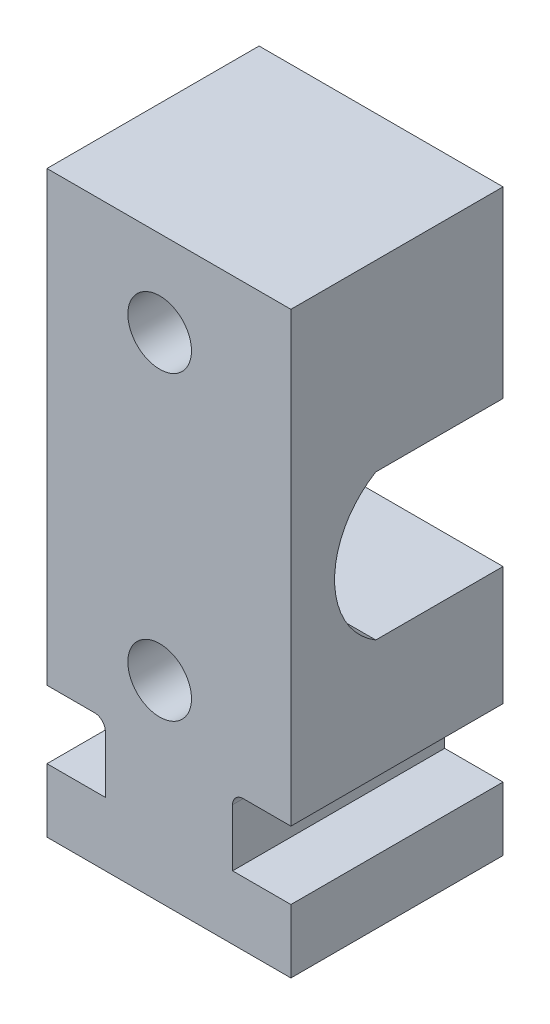
ISO-10303-21;
HEADER;
FILE_DESCRIPTION(('STEP AP214'),'2;1');
FILE_NAME('part.step','',(''),(''),'','','');
FILE_SCHEMA(('AUTOMOTIVE_DESIGN { 1 0 10303 214 1 1 1 1 }'));
ENDSEC;
DATA;
#1=APPLICATION_CONTEXT('core data for automotive mechanical design processes');
#2=APPLICATION_PROTOCOL_DEFINITION('international standard','automotive_design',2000,#1);
#3=PRODUCT_CONTEXT('',#1,'mechanical');
#4=PRODUCT('Part','Part','',(#3));
#5=PRODUCT_RELATED_PRODUCT_CATEGORY('part','',(#4));
#6=PRODUCT_DEFINITION_FORMATION('','',#4);
#7=PRODUCT_DEFINITION_CONTEXT('part definition',#1,'design');
#8=PRODUCT_DEFINITION('design','',#6,#7);
#9=PRODUCT_DEFINITION_SHAPE('','',#8);
#10=(LENGTH_UNIT() NAMED_UNIT(*) SI_UNIT(.MILLI.,.METRE.));
#11=(NAMED_UNIT(*) PLANE_ANGLE_UNIT() SI_UNIT($,.RADIAN.));
#12=(NAMED_UNIT(*) SI_UNIT($,.STERADIAN.) SOLID_ANGLE_UNIT());
#13=UNCERTAINTY_MEASURE_WITH_UNIT(LENGTH_MEASURE(1.E-05),#10,'distance_accuracy_value','');
#14=(GEOMETRIC_REPRESENTATION_CONTEXT(3) GLOBAL_UNCERTAINTY_ASSIGNED_CONTEXT((#13)) GLOBAL_UNIT_ASSIGNED_CONTEXT((#10,
#11,#12)) REPRESENTATION_CONTEXT('',''));
#15=CARTESIAN_POINT('',(0.,0.,0.));
#16=DIRECTION('',(0.,0.,1.));
#17=DIRECTION('',(1.,0.,0.));
#18=AXIS2_PLACEMENT_3D('',#15,#16,#17);
#19=CARTESIAN_POINT('',(115.,0.,100.));
#20=DIRECTION('',(-1.,0.,0.));
#21=DIRECTION('',(0.,0.,1.));
#22=AXIS2_PLACEMENT_3D('',#19,#20,#21);
#23=PLANE('',#22);
#24=DIRECTION('',(0.,0.,-1.));
#25=VECTOR('',#24,1.);
#26=CARTESIAN_POINT('',(115.,118.,100.));
#27=LINE('',#26,#25);
#28=CARTESIAN_POINT('',(115.,118.,60.));
#29=VERTEX_POINT('',#28);
#30=CARTESIAN_POINT('',(115.,118.,0.));
#31=VERTEX_POINT('',#30);
#32=EDGE_CURVE('E57',#29,#31,#27,.T.);
#33=ORIENTED_EDGE('',*,*,#32,.F.);
#34=CARTESIAN_POINT('',(115.,152.29480502863,39.4119853300948));
#35=DIRECTION('',(-1.,0.,0.));
#36=DIRECTION('',(0.,0.,1.));
#37=AXIS2_PLACEMENT_3D('',#34,#35,#36);
#38=CIRCLE('',#37,40.);
#39=CARTESIAN_POINT('',(115.,186.589610057261,60.));
#40=VERTEX_POINT('',#39);
#41=EDGE_CURVE('E58',#40,#29,#38,.F.);
#42=ORIENTED_EDGE('',*,*,#41,.F.);
#43=DIRECTION('',(0.,0.,1.));
#44=VECTOR('',#43,1.);
#45=CARTESIAN_POINT('',(115.,186.589610057261,100.));
#46=LINE('',#45,#44);
#47=CARTESIAN_POINT('',(115.,186.589610057261,0.));
#48=VERTEX_POINT('',#47);
#49=EDGE_CURVE('E180',#48,#40,#46,.T.);
#50=ORIENTED_EDGE('',*,*,#49,.F.);
#51=DIRECTION('',(0.,1.,0.));
#52=VECTOR('',#51,1.);
#53=CARTESIAN_POINT('',(115.,0.,0.));
#54=LINE('',#53,#52);
#55=CARTESIAN_POINT('',(115.,273.,0.));
#56=VERTEX_POINT('',#55);
#57=EDGE_CURVE('E165',#48,#56,#54,.T.);
#58=ORIENTED_EDGE('',*,*,#57,.T.);
#59=DIRECTION('',(0.,0.,-1.));
#60=VECTOR('',#59,1.);
#61=CARTESIAN_POINT('',(115.,273.,100.));
#62=LINE('',#61,#60);
#63=CARTESIAN_POINT('',(115.,273.,100.));
#64=VERTEX_POINT('',#63);
#65=EDGE_CURVE('E279',#64,#56,#62,.T.);
#66=ORIENTED_EDGE('',*,*,#65,.F.);
#67=DIRECTION('',(0.,1.,0.));
#68=VECTOR('',#67,1.);
#69=CARTESIAN_POINT('',(115.,0.,100.));
#70=LINE('',#69,#68);
#71=CARTESIAN_POINT('',(115.,62.,100.));
#72=VERTEX_POINT('',#71);
#73=EDGE_CURVE('E240',#72,#64,#70,.T.);
#74=ORIENTED_EDGE('',*,*,#73,.F.);
#75=DIRECTION('',(0.,0.,-1.));
#76=VECTOR('',#75,1.);
#77=CARTESIAN_POINT('',(115.,62.,100.));
#78=LINE('',#77,#76);
#79=CARTESIAN_POINT('',(115.,62.,0.));
#80=VERTEX_POINT('',#79);
#81=EDGE_CURVE('E278',#72,#80,#78,.T.);
#82=ORIENTED_EDGE('',*,*,#81,.T.);
#83=EDGE_CURVE('E172',#80,#31,#54,.T.);
#84=ORIENTED_EDGE('',*,*,#83,.T.);
#85=EDGE_LOOP('',(#33,#42,#50,#58,#66,#74,#82,#84));
#86=FACE_BOUND('',#85,.T.);
#87=ADVANCED_FACE('F41',(#86),#23,.F.);
#88=CARTESIAN_POINT('',(0.,0.,100.));
#89=DIRECTION('',(-1.,0.,0.));
#90=DIRECTION('',(0.,0.,1.));
#91=AXIS2_PLACEMENT_3D('',#88,#89,#90);
#92=PLANE('',#91);
#93=CARTESIAN_POINT('',(0.,152.29480502863,39.4119853300948));
#94=DIRECTION('',(-1.,0.,0.));
#95=DIRECTION('',(0.,0.,1.));
#96=AXIS2_PLACEMENT_3D('',#93,#94,#95);
#97=CIRCLE('',#96,40.);
#98=CARTESIAN_POINT('',(0.,186.589610057261,60.));
#99=VERTEX_POINT('',#98);
#100=CARTESIAN_POINT('',(0.,118.,60.));
#101=VERTEX_POINT('',#100);
#102=EDGE_CURVE('E11',#99,#101,#97,.F.);
#103=ORIENTED_EDGE('',*,*,#102,.T.);
#104=DIRECTION('',(0.,0.,-1.));
#105=VECTOR('',#104,1.);
#106=CARTESIAN_POINT('',(0.,118.,100.));
#107=LINE('',#106,#105);
#108=CARTESIAN_POINT('',(0.,118.,0.));
#109=VERTEX_POINT('',#108);
#110=EDGE_CURVE('E181',#101,#109,#107,.T.);
#111=ORIENTED_EDGE('',*,*,#110,.T.);
#112=DIRECTION('',(0.,1.,0.));
#113=VECTOR('',#112,1.);
#114=CARTESIAN_POINT('',(0.,0.,0.));
#115=LINE('',#114,#113);
#116=CARTESIAN_POINT('',(0.,62.,0.));
#117=VERTEX_POINT('',#116);
#118=EDGE_CURVE('E269',#117,#109,#115,.T.);
#119=ORIENTED_EDGE('',*,*,#118,.F.);
#120=DIRECTION('',(0.,0.,-1.));
#121=VECTOR('',#120,1.);
#122=CARTESIAN_POINT('',(0.,62.,100.));
#123=LINE('',#122,#121);
#124=CARTESIAN_POINT('',(0.,62.,100.));
#125=VERTEX_POINT('',#124);
#126=EDGE_CURVE('E274',#125,#117,#123,.T.);
#127=ORIENTED_EDGE('',*,*,#126,.F.);
#128=DIRECTION('',(0.,1.,0.));
#129=VECTOR('',#128,1.);
#130=CARTESIAN_POINT('',(0.,0.,100.));
#131=LINE('',#130,#129);
#132=CARTESIAN_POINT('',(0.,273.,100.));
#133=VERTEX_POINT('',#132);
#134=EDGE_CURVE('E237',#125,#133,#131,.T.);
#135=ORIENTED_EDGE('',*,*,#134,.T.);
#136=DIRECTION('',(0.,0.,-1.));
#137=VECTOR('',#136,1.);
#138=CARTESIAN_POINT('',(0.,273.,100.));
#139=LINE('',#138,#137);
#140=CARTESIAN_POINT('',(0.,273.,0.));
#141=VERTEX_POINT('',#140);
#142=EDGE_CURVE('E277',#133,#141,#139,.T.);
#143=ORIENTED_EDGE('',*,*,#142,.T.);
#144=CARTESIAN_POINT('',(0.,186.589610057261,0.));
#145=VERTEX_POINT('',#144);
#146=EDGE_CURVE('E267',#145,#141,#115,.T.);
#147=ORIENTED_EDGE('',*,*,#146,.F.);
#148=DIRECTION('',(0.,0.,1.));
#149=VECTOR('',#148,1.);
#150=CARTESIAN_POINT('',(0.,186.589610057261,100.));
#151=LINE('',#150,#149);
#152=EDGE_CURVE('E185',#145,#99,#151,.T.);
#153=ORIENTED_EDGE('',*,*,#152,.T.);
#154=EDGE_LOOP('',(#103,#111,#119,#127,#135,#143,#147,#153));
#155=FACE_BOUND('',#154,.T.);
#156=ADVANCED_FACE('F362',(#155),#92,.T.);
#157=CARTESIAN_POINT('',(0.,0.,0.));
#158=DIRECTION('',(0.,0.,1.));
#159=DIRECTION('',(1.,0.,0.));
#160=AXIS2_PLACEMENT_3D('',#157,#158,#159);
#161=PLANE('',#160);
#162=CARTESIAN_POINT('',(53.1264875684002,90.5995775376906,0.));
#163=DIRECTION('',(0.,0.,1.));
#164=DIRECTION('',(1.,0.,0.));
#165=AXIS2_PLACEMENT_3D('',#162,#163,#164);
#166=CIRCLE('',#165,15.);
#167=CARTESIAN_POINT('',(68.1264875684002,90.5995775376906,0.));
#168=VERTEX_POINT('',#167);
#169=EDGE_CURVE('E198',#168,#168,#166,.T.);
#170=ORIENTED_EDGE('',*,*,#169,.T.);
#171=EDGE_LOOP('',(#170));
#172=FACE_BOUND('',#171,.T.);
#173=DIRECTION('',(-1.,0.,0.));
#174=VECTOR('',#173,1.);
#175=CARTESIAN_POINT('',(0.,118.,0.));
#176=LINE('',#175,#174);
#177=EDGE_CURVE('E47',#31,#109,#176,.T.);
#178=ORIENTED_EDGE('',*,*,#177,.F.);
#179=ORIENTED_EDGE('',*,*,#83,.F.);
#180=DIRECTION('',(1.,0.,0.));
#181=VECTOR('',#180,1.);
#182=CARTESIAN_POINT('',(0.,62.,0.));
#183=LINE('',#182,#181);
#184=CARTESIAN_POINT('',(92.5,62.,0.));
#185=VERTEX_POINT('',#184);
#186=EDGE_CURVE('E174',#185,#80,#183,.T.);
#187=ORIENTED_EDGE('',*,*,#186,.F.);
#188=CARTESIAN_POINT('',(92.5,57.,0.));
#189=DIRECTION('',(0.,0.,1.));
#190=DIRECTION('',(1.,0.,0.));
#191=AXIS2_PLACEMENT_3D('',#188,#189,#190);
#192=CIRCLE('',#191,5.);
#193=CARTESIAN_POINT('',(87.5,57.,0.));
#194=VERTEX_POINT('',#193);
#195=EDGE_CURVE('E261',#194,#185,#192,.F.);
#196=ORIENTED_EDGE('',*,*,#195,.F.);
#197=DIRECTION('',(0.,1.,0.));
#198=VECTOR('',#197,1.);
#199=CARTESIAN_POINT('',(87.5,0.,0.));
#200=LINE('',#199,#198);
#201=CARTESIAN_POINT('',(87.5,30.,0.));
#202=VERTEX_POINT('',#201);
#203=EDGE_CURVE('E265',#202,#194,#200,.T.);
#204=ORIENTED_EDGE('',*,*,#203,.F.);
#205=DIRECTION('',(1.,0.,0.));
#206=VECTOR('',#205,1.);
#207=CARTESIAN_POINT('',(0.,30.,0.));
#208=LINE('',#207,#206);
#209=CARTESIAN_POINT('',(115.,30.,0.));
#210=VERTEX_POINT('',#209);
#211=EDGE_CURVE('E251',#202,#210,#208,.T.);
#212=ORIENTED_EDGE('',*,*,#211,.T.);
#213=DIRECTION('',(0.,1.,0.));
#214=VECTOR('',#213,1.);
#215=CARTESIAN_POINT('',(115.,0.,0.));
#216=LINE('',#215,#214);
#217=CARTESIAN_POINT('',(115.,0.,0.));
#218=VERTEX_POINT('',#217);
#219=EDGE_CURVE('E256',#218,#210,#216,.T.);
#220=ORIENTED_EDGE('',*,*,#219,.F.);
#221=DIRECTION('',(1.,0.,0.));
#222=VECTOR('',#221,1.);
#223=CARTESIAN_POINT('',(0.,0.,0.));
#224=LINE('',#223,#222);
#225=CARTESIAN_POINT('',(0.,0.,0.));
#226=VERTEX_POINT('',#225);
#227=EDGE_CURVE('E260',#226,#218,#224,.T.);
#228=ORIENTED_EDGE('',*,*,#227,.F.);
#229=DIRECTION('',(0.,1.,0.));
#230=VECTOR('',#229,1.);
#231=CARTESIAN_POINT('',(0.,0.,0.));
#232=LINE('',#231,#230);
#233=CARTESIAN_POINT('',(0.,30.,0.));
#234=VERTEX_POINT('',#233);
#235=EDGE_CURVE('E254',#226,#234,#232,.T.);
#236=ORIENTED_EDGE('',*,*,#235,.T.);
#237=CARTESIAN_POINT('',(27.5,30.,0.));
#238=VERTEX_POINT('',#237);
#239=EDGE_CURVE('E249',#234,#238,#208,.T.);
#240=ORIENTED_EDGE('',*,*,#239,.T.);
#241=DIRECTION('',(0.,1.,0.));
#242=VECTOR('',#241,1.);
#243=CARTESIAN_POINT('',(27.5,0.,0.));
#244=LINE('',#243,#242);
#245=CARTESIAN_POINT('',(27.5,57.,0.));
#246=VERTEX_POINT('',#245);
#247=EDGE_CURVE('E250',#238,#246,#244,.T.);
#248=ORIENTED_EDGE('',*,*,#247,.T.);
#249=CARTESIAN_POINT('',(22.5,57.,0.));
#250=DIRECTION('',(0.,0.,1.));
#251=DIRECTION('',(1.,0.,0.));
#252=AXIS2_PLACEMENT_3D('',#249,#250,#251);
#253=CIRCLE('',#252,5.);
#254=CARTESIAN_POINT('',(22.5,62.,0.));
#255=VERTEX_POINT('',#254);
#256=EDGE_CURVE('E203',#246,#255,#253,.T.);
#257=ORIENTED_EDGE('',*,*,#256,.T.);
#258=DIRECTION('',(-1.,0.,0.));
#259=VECTOR('',#258,1.);
#260=CARTESIAN_POINT('',(0.,62.,0.));
#261=LINE('',#260,#259);
#262=EDGE_CURVE('E220',#255,#117,#261,.T.);
#263=ORIENTED_EDGE('',*,*,#262,.T.);
#264=ORIENTED_EDGE('',*,*,#118,.T.);
#265=EDGE_LOOP('',(#178,#179,#187,#196,#204,#212,#220,#228,#236,#240,#248,#257,#263,#264));
#266=FACE_BOUND('',#265,.T.);
#267=ADVANCED_FACE('F309',(#172,#266),#161,.F.);
#268=CARTESIAN_POINT('',(53.1264875684002,232.599577537691,0.));
#269=DIRECTION('',(0.,0.,1.));
#270=DIRECTION('',(1.,0.,0.));
#271=AXIS2_PLACEMENT_3D('',#268,#269,#270);
#272=CIRCLE('',#271,15.);
#273=CARTESIAN_POINT('',(68.1264875684002,232.599577537691,0.));
#274=VERTEX_POINT('',#273);
#275=EDGE_CURVE('E201',#274,#274,#272,.T.);
#276=ORIENTED_EDGE('',*,*,#275,.T.);
#277=EDGE_LOOP('',(#276));
#278=FACE_BOUND('',#277,.T.);
#279=DIRECTION('',(1.,0.,0.));
#280=VECTOR('',#279,1.);
#281=CARTESIAN_POINT('',(-439.203527624976,186.589610057261,0.));
#282=LINE('',#281,#280);
#283=EDGE_CURVE('E166',#145,#48,#282,.T.);
#284=ORIENTED_EDGE('',*,*,#283,.F.);
#285=ORIENTED_EDGE('',*,*,#146,.T.);
#286=DIRECTION('',(1.,0.,0.));
#287=VECTOR('',#286,1.);
#288=CARTESIAN_POINT('',(-439.203527624976,273.,0.));
#289=LINE('',#288,#287);
#290=EDGE_CURVE('E171',#141,#56,#289,.T.);
#291=ORIENTED_EDGE('',*,*,#290,.T.);
#292=ORIENTED_EDGE('',*,*,#57,.F.);
#293=EDGE_LOOP('',(#284,#285,#291,#292));
#294=FACE_BOUND('',#293,.T.);
#295=ADVANCED_FACE('F164',(#278,#294),#161,.F.);
#296=CARTESIAN_POINT('',(22.5,57.,100.));
#297=DIRECTION('',(0.,0.,-1.));
#298=DIRECTION('',(-1.,0.,0.));
#299=AXIS2_PLACEMENT_3D('',#296,#297,#298);
#300=CYLINDRICAL_SURFACE('',#299,5.);
#301=ORIENTED_EDGE('',*,*,#256,.F.);
#302=DIRECTION('',(0.,0.,-1.));
#303=VECTOR('',#302,1.);
#304=CARTESIAN_POINT('',(27.5,57.,100.));
#305=LINE('',#304,#303);
#306=CARTESIAN_POINT('',(27.5,57.,100.));
#307=VERTEX_POINT('',#306);
#308=EDGE_CURVE('E305',#307,#246,#305,.T.);
#309=ORIENTED_EDGE('',*,*,#308,.F.);
#310=CARTESIAN_POINT('',(22.5,57.,100.));
#311=DIRECTION('',(0.,0.,1.));
#312=DIRECTION('',(1.,0.,0.));
#313=AXIS2_PLACEMENT_3D('',#310,#311,#312);
#314=CIRCLE('',#313,5.);
#315=CARTESIAN_POINT('',(22.5,62.,100.));
#316=VERTEX_POINT('',#315);
#317=EDGE_CURVE('E214',#307,#316,#314,.T.);
#318=ORIENTED_EDGE('',*,*,#317,.T.);
#319=DIRECTION('',(0.,0.,-1.));
#320=VECTOR('',#319,1.);
#321=CARTESIAN_POINT('',(22.5,62.,100.));
#322=LINE('',#321,#320);
#323=EDGE_CURVE('E242',#316,#255,#322,.T.);
#324=ORIENTED_EDGE('',*,*,#323,.T.);
#325=EDGE_LOOP('',(#301,#309,#318,#324));
#326=FACE_BOUND('',#325,.T.);
#327=ADVANCED_FACE('F43',(#326),#300,.F.);
#328=CARTESIAN_POINT('',(27.5,0.,100.));
#329=DIRECTION('',(-1.,0.,0.));
#330=DIRECTION('',(0.,0.,1.));
#331=AXIS2_PLACEMENT_3D('',#328,#329,#330);
#332=PLANE('',#331);
#333=ORIENTED_EDGE('',*,*,#247,.F.);
#334=DIRECTION('',(0.,0.,-1.));
#335=VECTOR('',#334,1.);
#336=CARTESIAN_POINT('',(27.5,30.,100.));
#337=LINE('',#336,#335);
#338=CARTESIAN_POINT('',(27.5,30.,100.));
#339=VERTEX_POINT('',#338);
#340=EDGE_CURVE('E297',#339,#238,#337,.T.);
#341=ORIENTED_EDGE('',*,*,#340,.F.);
#342=DIRECTION('',(0.,1.,0.));
#343=VECTOR('',#342,1.);
#344=CARTESIAN_POINT('',(27.5,0.,100.));
#345=LINE('',#344,#343);
#346=EDGE_CURVE('E217',#339,#307,#345,.T.);
#347=ORIENTED_EDGE('',*,*,#346,.T.);
#348=ORIENTED_EDGE('',*,*,#308,.T.);
#349=EDGE_LOOP('',(#333,#341,#347,#348));
#350=FACE_BOUND('',#349,.T.);
#351=ADVANCED_FACE('F355',(#350),#332,.T.);
#352=CARTESIAN_POINT('',(0.,30.,100.));
#353=DIRECTION('',(0.,1.,0.));
#354=DIRECTION('',(0.,0.,1.));
#355=AXIS2_PLACEMENT_3D('',#352,#353,#354);
#356=PLANE('',#355);
#357=ORIENTED_EDGE('',*,*,#239,.F.);
#358=DIRECTION('',(0.,0.,-1.));
#359=VECTOR('',#358,1.);
#360=CARTESIAN_POINT('',(0.,30.,100.));
#361=LINE('',#360,#359);
#362=CARTESIAN_POINT('',(0.,30.,100.));
#363=VERTEX_POINT('',#362);
#364=EDGE_CURVE('E296',#363,#234,#361,.T.);
#365=ORIENTED_EDGE('',*,*,#364,.F.);
#366=DIRECTION('',(1.,0.,0.));
#367=VECTOR('',#366,1.);
#368=CARTESIAN_POINT('',(0.,30.,100.));
#369=LINE('',#368,#367);
#370=EDGE_CURVE('E218',#363,#339,#369,.T.);
#371=ORIENTED_EDGE('',*,*,#370,.T.);
#372=ORIENTED_EDGE('',*,*,#340,.T.);
#373=EDGE_LOOP('',(#357,#365,#371,#372));
#374=FACE_BOUND('',#373,.T.);
#375=ADVANCED_FACE('F351',(#374),#356,.T.);
#376=CARTESIAN_POINT('',(0.,0.,100.));
#377=DIRECTION('',(-1.,0.,0.));
#378=DIRECTION('',(0.,0.,1.));
#379=AXIS2_PLACEMENT_3D('',#376,#377,#378);
#380=PLANE('',#379);
#381=ORIENTED_EDGE('',*,*,#235,.F.);
#382=DIRECTION('',(0.,0.,-1.));
#383=VECTOR('',#382,1.);
#384=CARTESIAN_POINT('',(0.,0.,100.));
#385=LINE('',#384,#383);
#386=CARTESIAN_POINT('',(0.,0.,100.));
#387=VERTEX_POINT('',#386);
#388=EDGE_CURVE('E298',#387,#226,#385,.T.);
#389=ORIENTED_EDGE('',*,*,#388,.F.);
#390=DIRECTION('',(0.,1.,0.));
#391=VECTOR('',#390,1.);
#392=CARTESIAN_POINT('',(0.,0.,100.));
#393=LINE('',#392,#391);
#394=EDGE_CURVE('E224',#387,#363,#393,.T.);
#395=ORIENTED_EDGE('',*,*,#394,.T.);
#396=ORIENTED_EDGE('',*,*,#364,.T.);
#397=EDGE_LOOP('',(#381,#389,#395,#396));
#398=FACE_BOUND('',#397,.T.);
#399=ADVANCED_FACE('F350',(#398),#380,.T.);
#400=CARTESIAN_POINT('',(0.,0.,100.));
#401=DIRECTION('',(0.,1.,0.));
#402=DIRECTION('',(0.,0.,1.));
#403=AXIS2_PLACEMENT_3D('',#400,#401,#402);
#404=PLANE('',#403);
#405=ORIENTED_EDGE('',*,*,#227,.T.);
#406=DIRECTION('',(0.,0.,-1.));
#407=VECTOR('',#406,1.);
#408=CARTESIAN_POINT('',(115.,0.,100.));
#409=LINE('',#408,#407);
#410=CARTESIAN_POINT('',(115.,0.,100.));
#411=VERTEX_POINT('',#410);
#412=EDGE_CURVE('E291',#411,#218,#409,.T.);
#413=ORIENTED_EDGE('',*,*,#412,.F.);
#414=DIRECTION('',(1.,0.,0.));
#415=VECTOR('',#414,1.);
#416=CARTESIAN_POINT('',(0.,0.,100.));
#417=LINE('',#416,#415);
#418=EDGE_CURVE('E227',#387,#411,#417,.T.);
#419=ORIENTED_EDGE('',*,*,#418,.F.);
#420=ORIENTED_EDGE('',*,*,#388,.T.);
#421=EDGE_LOOP('',(#405,#413,#419,#420));
#422=FACE_BOUND('',#421,.T.);
#423=ADVANCED_FACE('F341',(#422),#404,.F.);
#424=CARTESIAN_POINT('',(115.,0.,100.));
#425=DIRECTION('',(-1.,0.,0.));
#426=DIRECTION('',(0.,0.,1.));
#427=AXIS2_PLACEMENT_3D('',#424,#425,#426);
#428=PLANE('',#427);
#429=ORIENTED_EDGE('',*,*,#219,.T.);
#430=DIRECTION('',(0.,0.,-1.));
#431=VECTOR('',#430,1.);
#432=CARTESIAN_POINT('',(115.,30.,100.));
#433=LINE('',#432,#431);
#434=CARTESIAN_POINT('',(115.,30.,100.));
#435=VERTEX_POINT('',#434);
#436=EDGE_CURVE('E293',#435,#210,#433,.T.);
#437=ORIENTED_EDGE('',*,*,#436,.F.);
#438=DIRECTION('',(0.,1.,0.));
#439=VECTOR('',#438,1.);
#440=CARTESIAN_POINT('',(115.,0.,100.));
#441=LINE('',#440,#439);
#442=EDGE_CURVE('E230',#411,#435,#441,.T.);
#443=ORIENTED_EDGE('',*,*,#442,.F.);
#444=ORIENTED_EDGE('',*,*,#412,.T.);
#445=EDGE_LOOP('',(#429,#437,#443,#444));
#446=FACE_BOUND('',#445,.T.);
#447=ADVANCED_FACE('F339',(#446),#428,.F.);
#448=ORIENTED_EDGE('',*,*,#211,.F.);
#449=DIRECTION('',(0.,0.,-1.));
#450=VECTOR('',#449,1.);
#451=CARTESIAN_POINT('',(87.5,30.,100.));
#452=LINE('',#451,#450);
#453=CARTESIAN_POINT('',(87.5,30.,100.));
#454=VERTEX_POINT('',#453);
#455=EDGE_CURVE('E288',#454,#202,#452,.T.);
#456=ORIENTED_EDGE('',*,*,#455,.F.);
#457=EDGE_CURVE('E223',#454,#435,#369,.T.);
#458=ORIENTED_EDGE('',*,*,#457,.T.);
#459=ORIENTED_EDGE('',*,*,#436,.T.);
#460=EDGE_LOOP('',(#448,#456,#458,#459));
#461=FACE_BOUND('',#460,.T.);
#462=ADVANCED_FACE('F334',(#461),#356,.T.);
#463=CARTESIAN_POINT('',(87.5,0.,100.));
#464=DIRECTION('',(-1.,0.,0.));
#465=DIRECTION('',(0.,0.,1.));
#466=AXIS2_PLACEMENT_3D('',#463,#464,#465);
#467=PLANE('',#466);
#468=ORIENTED_EDGE('',*,*,#203,.T.);
#469=DIRECTION('',(0.,0.,-1.));
#470=VECTOR('',#469,1.);
#471=CARTESIAN_POINT('',(87.5,57.,100.));
#472=LINE('',#471,#470);
#473=CARTESIAN_POINT('',(87.5,57.,100.));
#474=VERTEX_POINT('',#473);
#475=EDGE_CURVE('E286',#474,#194,#472,.T.);
#476=ORIENTED_EDGE('',*,*,#475,.F.);
#477=DIRECTION('',(0.,1.,0.));
#478=VECTOR('',#477,1.);
#479=CARTESIAN_POINT('',(87.5,0.,100.));
#480=LINE('',#479,#478);
#481=EDGE_CURVE('E233',#454,#474,#480,.T.);
#482=ORIENTED_EDGE('',*,*,#481,.F.);
#483=ORIENTED_EDGE('',*,*,#455,.T.);
#484=EDGE_LOOP('',(#468,#476,#482,#483));
#485=FACE_BOUND('',#484,.T.);
#486=ADVANCED_FACE('F326',(#485),#467,.F.);
#487=CARTESIAN_POINT('',(92.5,57.,100.));
#488=DIRECTION('',(0.,0.,-1.));
#489=DIRECTION('',(-1.,0.,0.));
#490=AXIS2_PLACEMENT_3D('',#487,#488,#489);
#491=CYLINDRICAL_SURFACE('',#490,5.);
#492=ORIENTED_EDGE('',*,*,#195,.T.);
#493=DIRECTION('',(0.,0.,-1.));
#494=VECTOR('',#493,1.);
#495=CARTESIAN_POINT('',(92.5,62.,100.));
#496=LINE('',#495,#494);
#497=CARTESIAN_POINT('',(92.5,62.,100.));
#498=VERTEX_POINT('',#497);
#499=EDGE_CURVE('E284',#498,#185,#496,.T.);
#500=ORIENTED_EDGE('',*,*,#499,.F.);
#501=CARTESIAN_POINT('',(92.5,57.,100.));
#502=DIRECTION('',(0.,0.,1.));
#503=DIRECTION('',(1.,0.,0.));
#504=AXIS2_PLACEMENT_3D('',#501,#502,#503);
#505=CIRCLE('',#504,5.);
#506=EDGE_CURVE('E231',#474,#498,#505,.F.);
#507=ORIENTED_EDGE('',*,*,#506,.F.);
#508=ORIENTED_EDGE('',*,*,#475,.T.);
#509=EDGE_LOOP('',(#492,#500,#507,#508));
#510=FACE_BOUND('',#509,.T.);
#511=ADVANCED_FACE('F321',(#510),#491,.F.);
#512=CARTESIAN_POINT('',(0.,62.,100.));
#513=DIRECTION('',(0.,1.,0.));
#514=DIRECTION('',(0.,0.,1.));
#515=AXIS2_PLACEMENT_3D('',#512,#513,#514);
#516=PLANE('',#515);
#517=ORIENTED_EDGE('',*,*,#186,.T.);
#518=ORIENTED_EDGE('',*,*,#81,.F.);
#519=DIRECTION('',(1.,0.,0.));
#520=VECTOR('',#519,1.);
#521=CARTESIAN_POINT('',(0.,62.,100.));
#522=LINE('',#521,#520);
#523=EDGE_CURVE('E232',#498,#72,#522,.T.);
#524=ORIENTED_EDGE('',*,*,#523,.F.);
#525=ORIENTED_EDGE('',*,*,#499,.T.);
#526=EDGE_LOOP('',(#517,#518,#524,#525));
#527=FACE_BOUND('',#526,.T.);
#528=ADVANCED_FACE('F320',(#527),#516,.F.);
#529=CARTESIAN_POINT('',(0.,62.,100.));
#530=DIRECTION('',(0.,-1.,0.));
#531=DIRECTION('',(0.,0.,-1.));
#532=AXIS2_PLACEMENT_3D('',#529,#530,#531);
#533=PLANE('',#532);
#534=ORIENTED_EDGE('',*,*,#262,.F.);
#535=ORIENTED_EDGE('',*,*,#323,.F.);
#536=DIRECTION('',(-1.,0.,0.));
#537=VECTOR('',#536,1.);
#538=CARTESIAN_POINT('',(0.,62.,100.));
#539=LINE('',#538,#537);
#540=EDGE_CURVE('E241',#316,#125,#539,.T.);
#541=ORIENTED_EDGE('',*,*,#540,.T.);
#542=ORIENTED_EDGE('',*,*,#126,.T.);
#543=EDGE_LOOP('',(#534,#535,#541,#542));
#544=FACE_BOUND('',#543,.T.);
#545=ADVANCED_FACE('F363',(#544),#533,.T.);
#546=CARTESIAN_POINT('',(0.,0.,100.));
#547=DIRECTION('',(0.,0.,1.));
#548=DIRECTION('',(1.,0.,0.));
#549=AXIS2_PLACEMENT_3D('',#546,#547,#548);
#550=PLANE('',#549);
#551=ORIENTED_EDGE('',*,*,#506,.T.);
#552=ORIENTED_EDGE('',*,*,#523,.T.);
#553=ORIENTED_EDGE('',*,*,#73,.T.);
#554=DIRECTION('',(1.,0.,0.));
#555=VECTOR('',#554,1.);
#556=CARTESIAN_POINT('',(-439.203527624976,273.,100.));
#557=LINE('',#556,#555);
#558=EDGE_CURVE('E188',#133,#64,#557,.T.);
#559=ORIENTED_EDGE('',*,*,#558,.F.);
#560=ORIENTED_EDGE('',*,*,#134,.F.);
#561=ORIENTED_EDGE('',*,*,#540,.F.);
#562=ORIENTED_EDGE('',*,*,#317,.F.);
#563=ORIENTED_EDGE('',*,*,#346,.F.);
#564=ORIENTED_EDGE('',*,*,#370,.F.);
#565=ORIENTED_EDGE('',*,*,#394,.F.);
#566=ORIENTED_EDGE('',*,*,#418,.T.);
#567=ORIENTED_EDGE('',*,*,#442,.T.);
#568=ORIENTED_EDGE('',*,*,#457,.F.);
#569=ORIENTED_EDGE('',*,*,#481,.T.);
#570=EDGE_LOOP('',(#551,#552,#553,#559,#560,#561,#562,#563,#564,#565,#566,#567,#568,#569));
#571=FACE_BOUND('',#570,.T.);
#572=CARTESIAN_POINT('',(53.1264875684002,90.5995775376906,100.));
#573=DIRECTION('',(0.,0.,1.));
#574=DIRECTION('',(1.,0.,0.));
#575=AXIS2_PLACEMENT_3D('',#572,#573,#574);
#576=CIRCLE('',#575,15.);
#577=CARTESIAN_POINT('',(68.1264875684002,90.5995775376906,100.));
#578=VERTEX_POINT('',#577);
#579=EDGE_CURVE('E206',#578,#578,#576,.T.);
#580=ORIENTED_EDGE('',*,*,#579,.F.);
#581=EDGE_LOOP('',(#580));
#582=FACE_BOUND('',#581,.T.);
#583=CARTESIAN_POINT('',(53.1264875684002,232.599577537691,100.));
#584=DIRECTION('',(0.,0.,1.));
#585=DIRECTION('',(1.,0.,0.));
#586=AXIS2_PLACEMENT_3D('',#583,#584,#585);
#587=CIRCLE('',#586,15.);
#588=CARTESIAN_POINT('',(68.1264875684002,232.599577537691,100.));
#589=VERTEX_POINT('',#588);
#590=EDGE_CURVE('E205',#589,#589,#587,.T.);
#591=ORIENTED_EDGE('',*,*,#590,.F.);
#592=EDGE_LOOP('',(#591));
#593=FACE_BOUND('',#592,.T.);
#594=ADVANCED_FACE('F418',(#571,#582,#593),#550,.T.);
#595=CARTESIAN_POINT('',(53.1264875684002,90.5995775376906,0.));
#596=DIRECTION('',(0.,0.,1.));
#597=DIRECTION('',(1.,0.,0.));
#598=AXIS2_PLACEMENT_3D('',#595,#596,#597);
#599=CYLINDRICAL_SURFACE('',#598,15.);
#600=CARTESIAN_POINT('',(68.1264875684002,90.5995775376906,0.));
#601=CARTESIAN_POINT('',(68.1264875684002,90.5995775376906,1.04166666666666));
#602=CARTESIAN_POINT('',(68.1264875684002,90.5995775376906,2.08333333333333));
#603=CARTESIAN_POINT('',(68.1264875684002,90.5995775376906,4.16666666666667));
#604=CARTESIAN_POINT('',(68.1264875684002,90.5995775376906,5.20833333333333));
#605=CARTESIAN_POINT('',(68.1264875684002,90.5995775376906,7.29166666666667));
#606=CARTESIAN_POINT('',(68.1264875684002,90.5995775376906,8.33333333333333));
#607=CARTESIAN_POINT('',(68.1264875684002,90.5995775376906,10.4166666666667));
#608=CARTESIAN_POINT('',(68.1264875684002,90.5995775376906,11.4583333333333));
#609=CARTESIAN_POINT('',(68.1264875684002,90.5995775376906,13.5416666666667));
#610=CARTESIAN_POINT('',(68.1264875684002,90.5995775376906,14.5833333333333));
#611=CARTESIAN_POINT('',(68.1264875684002,90.5995775376906,16.6666666666667));
#612=CARTESIAN_POINT('',(68.1264875684002,90.5995775376906,17.7083333333333));
#613=CARTESIAN_POINT('',(68.1264875684002,90.5995775376906,19.7916666666667));
#614=CARTESIAN_POINT('',(68.1264875684002,90.5995775376906,20.8333333333333));
#615=CARTESIAN_POINT('',(68.1264875684002,90.5995775376906,22.9166666666667));
#616=CARTESIAN_POINT('',(68.1264875684002,90.5995775376906,23.9583333333333));
#617=CARTESIAN_POINT('',(68.1264875684002,90.5995775376906,26.0416666666667));
#618=CARTESIAN_POINT('',(68.1264875684002,90.5995775376906,27.0833333333333));
#619=CARTESIAN_POINT('',(68.1264875684002,90.5995775376906,29.1666666666667));
#620=CARTESIAN_POINT('',(68.1264875684002,90.5995775376906,30.2083333333333));
#621=CARTESIAN_POINT('',(68.1264875684002,90.5995775376906,32.2916666666667));
#622=CARTESIAN_POINT('',(68.1264875684002,90.5995775376906,33.3333333333333));
#623=CARTESIAN_POINT('',(68.1264875684002,90.5995775376906,35.4166666666667));
#624=CARTESIAN_POINT('',(68.1264875684002,90.5995775376906,36.4583333333333));
#625=CARTESIAN_POINT('',(68.1264875684002,90.5995775376906,38.5416666666667));
#626=CARTESIAN_POINT('',(68.1264875684002,90.5995775376906,39.5833333333333));
#627=CARTESIAN_POINT('',(68.1264875684002,90.5995775376906,41.6666666666667));
#628=CARTESIAN_POINT('',(68.1264875684002,90.5995775376906,42.7083333333333));
#629=CARTESIAN_POINT('',(68.1264875684002,90.5995775376906,44.7916666666667));
#630=CARTESIAN_POINT('',(68.1264875684002,90.5995775376906,45.8333333333333));
#631=CARTESIAN_POINT('',(68.1264875684002,90.5995775376906,47.9166666666667));
#632=CARTESIAN_POINT('',(68.1264875684002,90.5995775376906,48.9583333333333));
#633=CARTESIAN_POINT('',(68.1264875684002,90.5995775376906,51.0416666666667));
#634=CARTESIAN_POINT('',(68.1264875684002,90.5995775376906,52.0833333333333));
#635=CARTESIAN_POINT('',(68.1264875684002,90.5995775376906,54.1666666666667));
#636=CARTESIAN_POINT('',(68.1264875684002,90.5995775376906,55.2083333333333));
#637=CARTESIAN_POINT('',(68.1264875684002,90.5995775376906,57.2916666666667));
#638=CARTESIAN_POINT('',(68.1264875684002,90.5995775376906,58.3333333333333));
#639=CARTESIAN_POINT('',(68.1264875684002,90.5995775376906,60.4166666666667));
#640=CARTESIAN_POINT('',(68.1264875684002,90.5995775376906,61.4583333333333));
#641=CARTESIAN_POINT('',(68.1264875684002,90.5995775376906,63.5416666666667));
#642=CARTESIAN_POINT('',(68.1264875684002,90.5995775376906,64.5833333333333));
#643=CARTESIAN_POINT('',(68.1264875684002,90.5995775376906,66.6666666666667));
#644=CARTESIAN_POINT('',(68.1264875684002,90.5995775376906,67.7083333333333));
#645=CARTESIAN_POINT('',(68.1264875684002,90.5995775376906,69.7916666666667));
#646=CARTESIAN_POINT('',(68.1264875684002,90.5995775376906,70.8333333333333));
#647=CARTESIAN_POINT('',(68.1264875684002,90.5995775376906,72.9166666666667));
#648=CARTESIAN_POINT('',(68.1264875684002,90.5995775376906,73.9583333333333));
#649=CARTESIAN_POINT('',(68.1264875684002,90.5995775376906,76.0416666666667));
#650=CARTESIAN_POINT('',(68.1264875684002,90.5995775376906,77.0833333333333));
#651=CARTESIAN_POINT('',(68.1264875684002,90.5995775376906,79.1666666666666));
#652=CARTESIAN_POINT('',(68.1264875684002,90.5995775376906,80.2083333333333));
#653=CARTESIAN_POINT('',(68.1264875684002,90.5995775376906,82.2916666666667));
#654=CARTESIAN_POINT('',(68.1264875684002,90.5995775376906,83.3333333333333));
#655=CARTESIAN_POINT('',(68.1264875684002,90.5995775376906,85.4166666666667));
#656=CARTESIAN_POINT('',(68.1264875684002,90.5995775376906,86.4583333333333));
#657=CARTESIAN_POINT('',(68.1264875684002,90.5995775376906,88.5416666666667));
#658=CARTESIAN_POINT('',(68.1264875684002,90.5995775376906,89.5833333333333));
#659=CARTESIAN_POINT('',(68.1264875684002,90.5995775376906,91.6666666666667));
#660=CARTESIAN_POINT('',(68.1264875684002,90.5995775376906,92.7083333333333));
#661=CARTESIAN_POINT('',(68.1264875684002,90.5995775376906,94.7916666666666));
#662=CARTESIAN_POINT('',(68.1264875684002,90.5995775376906,95.8333333333333));
#663=CARTESIAN_POINT('',(68.1264875684002,90.5995775376906,97.9166666666667));
#664=CARTESIAN_POINT('',(68.1264875684002,90.5995775376906,98.9583333333333));
#665=CARTESIAN_POINT('',(68.1264875684002,90.5995775376906,100.));
#666=B_SPLINE_CURVE_WITH_KNOTS('',3,(#600,#601,#602,#603,#604,#605,#606,#607,#608,#609,#610,
#611,#612,#613,#614,#615,#616,#617,#618,#619,#620,#621,#622,#623,#624,#625,#626,#627,#628,#629,
#630,#631,#632,#633,#634,#635,#636,#637,#638,#639,#640,#641,#642,#643,#644,#645,#646,#647,#648,
#649,#650,#651,#652,#653,#654,#655,#656,#657,#658,#659,#660,#661,#662,#663,#664,#665),
.UNSPECIFIED.,.F.,.F.,(4,2,2,2,2,2,2,2,2,2,2,2,2,2,2,2,2,2,2,2,2,2,2,2,2,2,2,2,2,2,2,2,4),(0.,
3.125,6.25,9.375,12.5,15.625,18.75,21.875,25.,28.125,31.25,34.375,37.5,40.625,43.75,46.875,50.,
53.125,56.25,59.375,62.5,65.625,68.75,71.875,75.,78.125,81.25,84.375,87.5,90.625,93.75,96.875,
100.),.UNSPECIFIED.);
#667=EDGE_CURVE('BSEAM424',#168,#578,#666,.T.);
#668=ORIENTED_EDGE('',*,*,#169,.F.);
#669=ORIENTED_EDGE('',*,*,#579,.T.);
#670=ORIENTED_EDGE('',*,*,#667,.T.);
#671=ORIENTED_EDGE('',*,*,#667,.F.);
#672=EDGE_LOOP('',(#668,#670,#669,#671));
#673=FACE_BOUND('',#672,.T.);
#674=ADVANCED_FACE('F424',(#673),#599,.F.);
#675=CARTESIAN_POINT('',(53.1264875684002,232.599577537691,0.));
#676=DIRECTION('',(0.,0.,1.));
#677=DIRECTION('',(1.,0.,0.));
#678=AXIS2_PLACEMENT_3D('',#675,#676,#677);
#679=CYLINDRICAL_SURFACE('',#678,15.);
#680=CARTESIAN_POINT('',(68.1264875684002,232.599577537691,0.));
#681=CARTESIAN_POINT('',(68.1264875684002,232.599577537691,1.04166666666666));
#682=CARTESIAN_POINT('',(68.1264875684002,232.599577537691,2.08333333333333));
#683=CARTESIAN_POINT('',(68.1264875684002,232.599577537691,4.16666666666667));
#684=CARTESIAN_POINT('',(68.1264875684002,232.599577537691,5.20833333333333));
#685=CARTESIAN_POINT('',(68.1264875684002,232.599577537691,7.29166666666667));
#686=CARTESIAN_POINT('',(68.1264875684002,232.599577537691,8.33333333333333));
#687=CARTESIAN_POINT('',(68.1264875684002,232.599577537691,10.4166666666667));
#688=CARTESIAN_POINT('',(68.1264875684002,232.599577537691,11.4583333333333));
#689=CARTESIAN_POINT('',(68.1264875684002,232.599577537691,13.5416666666667));
#690=CARTESIAN_POINT('',(68.1264875684002,232.599577537691,14.5833333333333));
#691=CARTESIAN_POINT('',(68.1264875684002,232.599577537691,16.6666666666667));
#692=CARTESIAN_POINT('',(68.1264875684002,232.599577537691,17.7083333333333));
#693=CARTESIAN_POINT('',(68.1264875684002,232.599577537691,19.7916666666667));
#694=CARTESIAN_POINT('',(68.1264875684002,232.599577537691,20.8333333333333));
#695=CARTESIAN_POINT('',(68.1264875684002,232.599577537691,22.9166666666667));
#696=CARTESIAN_POINT('',(68.1264875684002,232.599577537691,23.9583333333333));
#697=CARTESIAN_POINT('',(68.1264875684002,232.599577537691,26.0416666666667));
#698=CARTESIAN_POINT('',(68.1264875684002,232.599577537691,27.0833333333333));
#699=CARTESIAN_POINT('',(68.1264875684002,232.599577537691,29.1666666666667));
#700=CARTESIAN_POINT('',(68.1264875684002,232.599577537691,30.2083333333333));
#701=CARTESIAN_POINT('',(68.1264875684002,232.599577537691,32.2916666666667));
#702=CARTESIAN_POINT('',(68.1264875684002,232.599577537691,33.3333333333333));
#703=CARTESIAN_POINT('',(68.1264875684002,232.599577537691,35.4166666666667));
#704=CARTESIAN_POINT('',(68.1264875684002,232.599577537691,36.4583333333333));
#705=CARTESIAN_POINT('',(68.1264875684002,232.599577537691,38.5416666666667));
#706=CARTESIAN_POINT('',(68.1264875684002,232.599577537691,39.5833333333333));
#707=CARTESIAN_POINT('',(68.1264875684002,232.599577537691,41.6666666666667));
#708=CARTESIAN_POINT('',(68.1264875684002,232.599577537691,42.7083333333333));
#709=CARTESIAN_POINT('',(68.1264875684002,232.599577537691,44.7916666666667));
#710=CARTESIAN_POINT('',(68.1264875684002,232.599577537691,45.8333333333333));
#711=CARTESIAN_POINT('',(68.1264875684002,232.599577537691,47.9166666666667));
#712=CARTESIAN_POINT('',(68.1264875684002,232.599577537691,48.9583333333333));
#713=CARTESIAN_POINT('',(68.1264875684002,232.599577537691,51.0416666666667));
#714=CARTESIAN_POINT('',(68.1264875684002,232.599577537691,52.0833333333333));
#715=CARTESIAN_POINT('',(68.1264875684002,232.599577537691,54.1666666666667));
#716=CARTESIAN_POINT('',(68.1264875684002,232.599577537691,55.2083333333333));
#717=CARTESIAN_POINT('',(68.1264875684002,232.599577537691,57.2916666666667));
#718=CARTESIAN_POINT('',(68.1264875684002,232.599577537691,58.3333333333333));
#719=CARTESIAN_POINT('',(68.1264875684002,232.599577537691,60.4166666666667));
#720=CARTESIAN_POINT('',(68.1264875684002,232.599577537691,61.4583333333333));
#721=CARTESIAN_POINT('',(68.1264875684002,232.599577537691,63.5416666666667));
#722=CARTESIAN_POINT('',(68.1264875684002,232.599577537691,64.5833333333333));
#723=CARTESIAN_POINT('',(68.1264875684002,232.599577537691,66.6666666666667));
#724=CARTESIAN_POINT('',(68.1264875684002,232.599577537691,67.7083333333333));
#725=CARTESIAN_POINT('',(68.1264875684002,232.599577537691,69.7916666666667));
#726=CARTESIAN_POINT('',(68.1264875684002,232.599577537691,70.8333333333333));
#727=CARTESIAN_POINT('',(68.1264875684002,232.599577537691,72.9166666666667));
#728=CARTESIAN_POINT('',(68.1264875684002,232.599577537691,73.9583333333333));
#729=CARTESIAN_POINT('',(68.1264875684002,232.599577537691,76.0416666666667));
#730=CARTESIAN_POINT('',(68.1264875684002,232.599577537691,77.0833333333333));
#731=CARTESIAN_POINT('',(68.1264875684002,232.599577537691,79.1666666666666));
#732=CARTESIAN_POINT('',(68.1264875684002,232.599577537691,80.2083333333333));
#733=CARTESIAN_POINT('',(68.1264875684002,232.599577537691,82.2916666666667));
#734=CARTESIAN_POINT('',(68.1264875684002,232.599577537691,83.3333333333333));
#735=CARTESIAN_POINT('',(68.1264875684002,232.599577537691,85.4166666666667));
#736=CARTESIAN_POINT('',(68.1264875684002,232.599577537691,86.4583333333333));
#737=CARTESIAN_POINT('',(68.1264875684002,232.599577537691,88.5416666666667));
#738=CARTESIAN_POINT('',(68.1264875684002,232.599577537691,89.5833333333333));
#739=CARTESIAN_POINT('',(68.1264875684002,232.599577537691,91.6666666666667));
#740=CARTESIAN_POINT('',(68.1264875684002,232.599577537691,92.7083333333333));
#741=CARTESIAN_POINT('',(68.1264875684002,232.599577537691,94.7916666666666));
#742=CARTESIAN_POINT('',(68.1264875684002,232.599577537691,95.8333333333333));
#743=CARTESIAN_POINT('',(68.1264875684002,232.599577537691,97.9166666666667));
#744=CARTESIAN_POINT('',(68.1264875684002,232.599577537691,98.9583333333333));
#745=CARTESIAN_POINT('',(68.1264875684002,232.599577537691,100.));
#746=B_SPLINE_CURVE_WITH_KNOTS('',3,(#680,#681,#682,#683,#684,#685,#686,#687,#688,#689,#690,
#691,#692,#693,#694,#695,#696,#697,#698,#699,#700,#701,#702,#703,#704,#705,#706,#707,#708,#709,
#710,#711,#712,#713,#714,#715,#716,#717,#718,#719,#720,#721,#722,#723,#724,#725,#726,#727,#728,
#729,#730,#731,#732,#733,#734,#735,#736,#737,#738,#739,#740,#741,#742,#743,#744,#745),
.UNSPECIFIED.,.F.,.F.,(4,2,2,2,2,2,2,2,2,2,2,2,2,2,2,2,2,2,2,2,2,2,2,2,2,2,2,2,2,2,2,2,4),(0.,
3.125,6.25,9.375,12.5,15.625,18.75,21.875,25.,28.125,31.25,34.375,37.5,40.625,43.75,46.875,50.,
53.125,56.25,59.375,62.5,65.625,68.75,71.875,75.,78.125,81.25,84.375,87.5,90.625,93.75,96.875,
100.),.UNSPECIFIED.);
#747=EDGE_CURVE('BSEAM380',#274,#589,#746,.T.);
#748=ORIENTED_EDGE('',*,*,#275,.F.);
#749=ORIENTED_EDGE('',*,*,#590,.T.);
#750=ORIENTED_EDGE('',*,*,#747,.T.);
#751=ORIENTED_EDGE('',*,*,#747,.F.);
#752=EDGE_LOOP('',(#748,#750,#749,#751));
#753=FACE_BOUND('',#752,.T.);
#754=ADVANCED_FACE('F380',(#753),#679,.F.);
#755=CARTESIAN_POINT('',(-439.203527624976,273.,0.));
#756=DIRECTION('',(0.,1.,0.));
#757=DIRECTION('',(0.,0.,1.));
#758=AXIS2_PLACEMENT_3D('',#755,#756,#757);
#759=PLANE('',#758);
#760=ORIENTED_EDGE('',*,*,#65,.T.);
#761=ORIENTED_EDGE('',*,*,#290,.F.);
#762=ORIENTED_EDGE('',*,*,#142,.F.);
#763=ORIENTED_EDGE('',*,*,#558,.T.);
#764=EDGE_LOOP('',(#760,#761,#762,#763));
#765=FACE_BOUND('',#764,.T.);
#766=ADVANCED_FACE('F369',(#765),#759,.T.);
#767=CARTESIAN_POINT('',(-439.203527624976,152.29480502863,39.4119853300948));
#768=DIRECTION('',(1.,0.,0.));
#769=DIRECTION('',(0.,0.,-1.));
#770=AXIS2_PLACEMENT_3D('',#767,#768,#769);
#771=CYLINDRICAL_SURFACE('',#770,40.);
#772=DIRECTION('',(1.,0.,0.));
#773=VECTOR('',#772,1.);
#774=CARTESIAN_POINT('',(-439.203527624976,186.589610057261,60.));
#775=LINE('',#774,#773);
#776=EDGE_CURVE('E187',#99,#40,#775,.T.);
#777=ORIENTED_EDGE('',*,*,#776,.T.);
#778=ORIENTED_EDGE('',*,*,#41,.T.);
#779=DIRECTION('',(1.,0.,0.));
#780=VECTOR('',#779,1.);
#781=CARTESIAN_POINT('',(-439.203527624976,118.,60.));
#782=LINE('',#781,#780);
#783=EDGE_CURVE('E189',#101,#29,#782,.T.);
#784=ORIENTED_EDGE('',*,*,#783,.F.);
#785=ORIENTED_EDGE('',*,*,#102,.F.);
#786=EDGE_LOOP('',(#777,#778,#784,#785));
#787=FACE_BOUND('',#786,.T.);
#788=ADVANCED_FACE('F368',(#787),#771,.F.);
#789=CARTESIAN_POINT('',(-439.203527624976,118.,60.));
#790=DIRECTION('',(0.,1.,0.));
#791=DIRECTION('',(0.,0.,1.));
#792=AXIS2_PLACEMENT_3D('',#789,#790,#791);
#793=PLANE('',#792);
#794=ORIENTED_EDGE('',*,*,#783,.T.);
#795=ORIENTED_EDGE('',*,*,#32,.T.);
#796=ORIENTED_EDGE('',*,*,#177,.T.);
#797=ORIENTED_EDGE('',*,*,#110,.F.);
#798=EDGE_LOOP('',(#794,#795,#796,#797));
#799=FACE_BOUND('',#798,.T.);
#800=ADVANCED_FACE('F306',(#799),#793,.T.);
#801=CARTESIAN_POINT('',(-439.203527624976,186.589610057261,0.));
#802=DIRECTION('',(0.,-1.,0.));
#803=DIRECTION('',(0.,0.,-1.));
#804=AXIS2_PLACEMENT_3D('',#801,#802,#803);
#805=PLANE('',#804);
#806=ORIENTED_EDGE('',*,*,#283,.T.);
#807=ORIENTED_EDGE('',*,*,#49,.T.);
#808=ORIENTED_EDGE('',*,*,#776,.F.);
#809=ORIENTED_EDGE('',*,*,#152,.F.);
#810=EDGE_LOOP('',(#806,#807,#808,#809));
#811=FACE_BOUND('',#810,.T.);
#812=ADVANCED_FACE('F184',(#811),#805,.T.);
#813=CLOSED_SHELL('',(#87,#156,#267,#295,#327,#351,#375,#399,#423,#447,#462,#486,#511,#528,#545,
#594,#674,#754,#766,#788,#800,#812));
#814=MANIFOLD_SOLID_BREP('B2',#813);
#815=ADVANCED_BREP_SHAPE_REPRESENTATION('',(#18,#814),#14);
#816=SHAPE_DEFINITION_REPRESENTATION(#9,#815);
ENDSEC;
END-ISO-10303-21;
